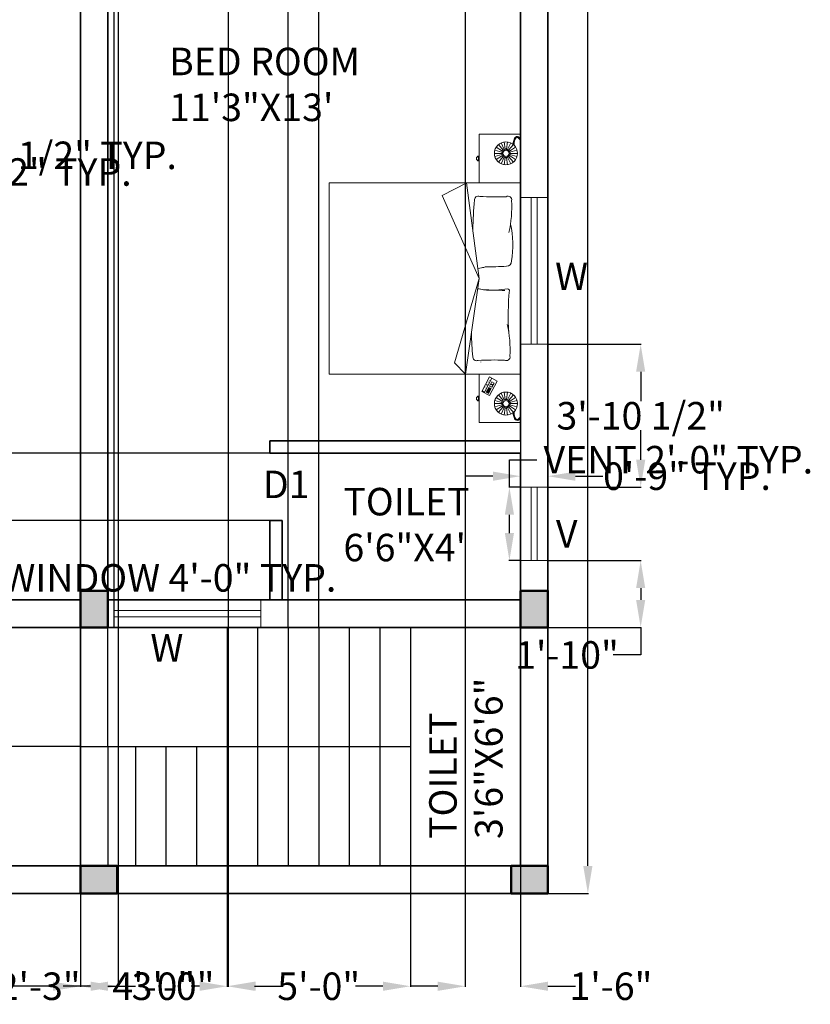
# Model space of a CAD drawing. Units: inches. Extents: x 113 to 575, y 111 to 799.
# Tile 2 of 4: x 317 to 575, y 119 to 441. Entities that reach past the tile are written whole.
import ezdxf

# ---------------------------------------------------------------- set-up
doc = ezdxf.new("R2010")
doc.units = ezdxf.units.IN
doc.header["$MEASUREMENT"] = 0
for name, color, linetype, lineweight in [('A-ANNO-DIMS', 2, 'Continuous', 18), ('A-ANNO-TEXT', 7, 'Continuous', 18), ('A-AREA-IDEN', 7, 'Continuous', 25), ('A-COLS', 7, 'Continuous', 50), ('A-COLS-PATT', 252, 'Continuous', 13), ('A-FLOR-STRS', 7, 'Continuous', 25), ('A-FURN', 8, 'Continuous', 18), ('A-GLAZ', 4, 'Continuous', 18), ('A-WALL', 7, 'Continuous', 35)]:
    doc.layers.add(name, color=color, linetype=linetype, lineweight=lineweight)
doc.styles.get("Standard").update_dxf_attribs({"font": 'arial.ttf'})
doc.dimstyles.get("Standard").update_dxf_attribs({"dimtxt": 9, "dimasz": 9, "dimexe": 0.18, "dimexo": 0.0625, "dimgap": 0.09, "dimtad": 0, "dimtih": 1, "dimtoh": 1, "dimdec": 0, "dimzin": 0, "dimdsep": 46, "dimlunit": 3, "dimtxsty": 'Standard', "dimcen": 0.09, "dimadec": 0, "dimazin": 0, "dimtfac": 1, "dimtdec": 0, "dimtofl": 0, "dimtmove": 0, "dimatfit": 3, "dimfxl": 1, "dimtolj": 1, "dimtzin": 0, "dimarcsym": 0})

# ---------------------------------------------------------------- blocks, each defined once
blk = doc.blocks.new('23')
for p, q in [((198.0513, 218.5507), (197.5897, 218.5507)), ((197.5897, 218.5507), (197.5897, 218.1608)), ((198.0513, 218.5507), (197.5897, 218.5507)), ((197.7114, 218.5049), (197.7492, 218.4461)), ((197.7398, 218.5179), (197.7595, 218.4508)), ((197.7707, 218.5223), (197.7707, 218.4524)), ((197.7707, 218.5223), (197.7707, 218.4524)), ((197.8016, 218.5179), (197.7819, 218.4508)), ((197.7922, 218.4461), (197.83, 218.5049)), ((198.0513, 216.7325), (198.0513, 218.5507)), ((198.0513, 218.5507), (198.9604, 218.5507)), ((198.0513, 218.5507), (199.8695, 218.5507)), ((198.0513, 218.5507), (198.0513, 218.1608)), ((199.8695, 218.5507), (200.3311, 218.5507)), ((199.8695, 218.5507), (200.3311, 218.5507)), ((199.8695, 218.5507), (199.8695, 216.7325)), ((200.1286, 218.4461), (200.0908, 218.5049)), ((200.1191, 218.5179), (200.1388, 218.4508)), ((200.15, 218.5223), (200.15, 218.4524)), ((200.15, 218.5223), (200.15, 218.4524)), ((200.1809, 218.5179), (200.1612, 218.4508)), ((200.2093, 218.5049), (200.1715, 218.4461)), ((200.3311, 218.5507), (200.3311, 218.1608)), ((197.6622, 218.4283), (197.7314, 218.4183)), ((197.6622, 218.3971), (197.7314, 218.407)), ((197.671, 218.4582), (197.7346, 218.4292)), ((197.671, 218.3671), (197.7346, 218.3962)), ((197.6878, 218.4845), (197.7407, 218.4387)), ((197.742, 218.419), (197.7324, 218.4232)), ((197.744, 218.425), (197.7336, 218.4267)), ((197.7863, 218.4377), (197.7953, 218.4438)), ((197.7934, 218.4314), (197.7991, 218.4404)), ((197.8007, 218.4387), (197.8536, 218.4845)), ((197.8068, 218.4292), (197.8704, 218.4582)), ((197.8068, 218.3962), (197.8704, 218.3671)), ((197.81, 218.4183), (197.8792, 218.4283)), ((197.81, 218.407), (197.8792, 218.3971)), ((200.1107, 218.4183), (200.0415, 218.4283)), ((200.1107, 218.407), (200.0415, 218.3971)), ((200.1139, 218.4292), (200.0503, 218.4582)), ((200.1139, 218.3962), (200.0503, 218.3671)), ((200.12, 218.4387), (200.0672, 218.4845)), ((200.1273, 218.4314), (200.1216, 218.4404)), ((200.1345, 218.4377), (200.1254, 218.4438)), ((200.1768, 218.425), (200.1872, 218.4267)), ((200.1788, 218.419), (200.1883, 218.4232)), ((200.2329, 218.4845), (200.18, 218.4387)), ((200.2498, 218.4582), (200.1862, 218.4292)), ((200.2498, 218.3671), (200.1862, 218.3962)), ((200.2586, 218.4283), (200.1893, 218.4183)), ((200.2586, 218.3971), (200.1893, 218.407)), ((197.6878, 218.3409), (197.7407, 218.3867)), ((197.7114, 218.3204), (197.7492, 218.3793)), ((197.7595, 218.3746), (197.7398, 218.3075)), ((197.7654, 218.3837), (197.7654, 218.3733)), ((197.7722, 218.3833), (197.7696, 218.373)), ((197.7707, 218.373), (197.7707, 218.303)), ((197.7707, 218.373), (197.7707, 218.303)), ((197.7819, 218.3746), (197.8016, 218.3075)), ((197.7922, 218.3793), (197.83, 218.3204)), ((197.8007, 218.3867), (197.8536, 218.3409)), ((199.897, 218.2553), (199.9365, 218.3298)), ((199.9365, 218.3298), (200.0738, 218.257)), ((200.12, 218.3867), (200.0672, 218.3409)), ((200.1286, 218.3793), (200.0908, 218.3204)), ((200.1388, 218.3746), (200.1191, 218.3075)), ((200.1486, 218.3833), (200.1512, 218.373)), ((200.15, 218.373), (200.15, 218.303)), ((200.15, 218.373), (200.15, 218.303)), ((200.1554, 218.3837), (200.1553, 218.3733)), ((200.1612, 218.3746), (200.1809, 218.3075)), ((200.2093, 218.3204), (200.1715, 218.3793)), ((200.2329, 218.3409), (200.18, 218.3867)), ((200.0344, 218.1825), (199.897, 218.2553)), ((199.9093, 218.2786), (200.0467, 218.2057)), ((199.9435, 218.2784), (199.9546, 218.2994)), ((199.9608, 218.2692), (199.9435, 218.2784)), ((199.9546, 218.2994), (199.972, 218.2902)), ((199.972, 218.2902), (199.9608, 218.2692)), ((199.9658, 218.2665), (199.977, 218.2875)), ((199.9832, 218.2573), (199.9658, 218.2665)), ((199.977, 218.2875), (199.9943, 218.2783)), ((199.9943, 218.2783), (199.9832, 218.2573)), ((199.9967, 218.2502), (200.0078, 218.2711)), ((200.0421, 218.2261), (199.9967, 218.2502)), ((200.044, 218.2298), (199.9986, 218.2538)), ((200.0458, 218.2332), (200.0004, 218.2572)), ((200.0469, 218.2353), (200.0016, 218.2594)), ((200.0482, 218.2378), (200.0029, 218.2618)), ((200.0498, 218.2406), (200.0044, 218.2647)), ((200.0519, 218.2446), (200.0065, 218.2687)), ((200.0532, 218.2471), (200.0078, 218.2711)), ((200.0738, 218.257), (200.0344, 218.1825)), ((200.0532, 218.2471), (200.0421, 218.2261)), ((197.5921, 218.1584), (198.0489, 218.1584)), ((197.7986, 218.1491), (197.7986, 218.1437)), ((197.84, 218.1515), (197.801, 218.1515)), ((197.801, 218.1413), (197.8052, 218.1413)), ((197.8076, 218.1389), (197.8076, 218.135)), ((197.81, 218.1326), (197.8309, 218.1326)), ((197.8286, 218.1584), (197.8124, 218.1584)), ((197.8124, 218.1584), (197.8124, 218.1515)), ((197.8286, 218.1515), (197.8286, 218.1584)), ((197.8333, 218.135), (197.8333, 218.1413)), ((197.8333, 218.1413), (197.84, 218.1413)), ((197.8424, 218.1437), (197.8424, 218.1491)), ((198.9604, 218.1582), (198.0513, 218.039)), ((198.171, 217.8058), (198.9604, 218.1582)), ((199.763, 217.9219), (198.9604, 218.1582)), ((198.9604, 218.1582), (199.8695, 218.0282)), ((200.3287, 218.1584), (199.8719, 218.1584)), ((200.0784, 218.1437), (200.0784, 218.1491)), ((200.0808, 218.1515), (200.1197, 218.1515)), ((200.0874, 218.1413), (200.0808, 218.1413)), ((200.0874, 218.135), (200.0874, 218.1413)), ((200.1107, 218.1326), (200.0898, 218.1326)), ((200.0922, 218.1515), (200.0922, 218.1584)), ((200.0922, 218.1584), (200.1084, 218.1584)), ((200.1084, 218.1584), (200.1084, 218.1515)), ((200.1131, 218.1389), (200.1131, 218.135)), ((200.1197, 218.1413), (200.1155, 218.1413)), ((200.1221, 218.1491), (200.1221, 218.1437)), ((198.0513, 218.042), (198.171, 217.8058)), ((199.8695, 218.0282), (199.763, 217.9219)), ((198.9604, 216.7325), (198.0513, 216.7325)), ((198.9604, 216.7325), (199.8695, 216.7325))]:
    blk.add_line(p, q)
for centre, radius in [((197.7707, 218.4127), 0.1096), ((200.15, 218.4127), 0.1096), ((197.7707, 218.4127), 0.0397), ((197.7707, 218.4127), 0.0294), ((200.15, 218.4127), 0.0397), ((200.15, 218.4127), 0.0294)]:
    blk.add_circle(centre, radius)
for centre, radius, start, end in [((198.2131, 218.4327), 0.035, 78.72779, 211.6095), ((198.2131, 218.4327), 0.035, 78.72779, 211.6095), ((194.5801, 218.3261), 3.6043, 357.43333, 1.40375), ((194.5801, 218.3261), 3.6043, 357.43333, 1.40375), ((198.2779, 217.3787), 1.0899, 77.05638, 93.04883), ((198.2779, 217.3787), 1.0899, 77.05638, 93.04883), ((198.6485, 217.4959), 0.982, 81.47023, 102.10326), ((198.6485, 217.4959), 0.982, 81.47023, 102.10326), ((198.7941, 218.4167), 0.0503, 0, 90), ((198.7941, 218.4167), 0.0503, 0, 90), ((192.8563, 218.1202), 5.9955, 0.91256, 2.83406), ((192.8563, 218.1202), 5.9955, 0.91256, 2.83406), ((199.1058, 218.4025), 0.0559, 128.22652, 148.49477), ((198.0818, 218.2709), 0.9895, 355.87807, 9.3556), ((205.0634, 218.1043), 5.9955, 177.16594, 179.08744), ((199.3105, 220.7603), 2.3262, 264.09622, 274.11018), ((199.1058, 218.4025), 0.0559, 41.3461, 41.8512), ((199.6418, 217.3627), 1.0899, 86.95117, 102.94362), ((199.6418, 217.3627), 1.0899, 86.95117, 102.94362), ((199.7066, 218.4167), 0.035, 328.3905, 101.27221), ((199.7066, 218.4167), 0.035, 328.3905, 101.27221), ((203.3397, 218.3101), 3.6043, 178.59625, 182.56667), ((203.3397, 218.3101), 3.6043, 178.59625, 182.56667), ((198.7853, 218.1859), 0.0722, 2.66977, 24.37437), ((198.5509, 218.1138), 0.3169, 5.86257, 18.75888), ((199.968, 218.2279), 0.00141, 90, 270), ((199.968, 218.2279), 0.00141, 270, 90), ((199.9724, 218.235), 0.00141, 90, 270), ((199.9724, 218.235), 0.00141, 270, 90), ((197.5921, 218.1608), 0.0024, 180, 270), ((197.801, 218.1491), 0.0024, 90, 180), ((197.801, 218.1437), 0.0024, 180, 270), ((197.8052, 218.1389), 0.0024, 0, 90), ((197.81, 218.135), 0.0024, 180, 270), ((197.8309, 218.135), 0.0024, 270, 0), ((197.84, 218.1491), 0.0024, 0, 90), ((197.84, 218.1437), 0.0024, 270, 0), ((198.2139, 218.15), 0.0362, 156.10841, 279.65758), ((198.2139, 218.15), 0.0362, 156.10841, 279.65758), ((198.5015, 220.904), 2.805, 264.11391, 269.91574), ((198.5015, 220.904), 2.805, 264.11391, 269.91574), ((199.1999, 218.1498), 0.1404, 159.16323, 182.37479), ((199.1345, 218.17), 0.0722, 155.62563, 177.33023), ((199.7059, 218.134), 0.0362, 260.34242, 23.89159), ((199.7059, 218.134), 0.0362, 260.34242, 23.89159), ((199.755, 218.1754), 0.00192, 180, 270), ((200.0315, 218.1913), 0.00141, 90, 270), ((200.0315, 218.1913), 0.00141, 270, 90), ((200.0366, 218.2002), 0.00141, 90, 270), ((200.0366, 218.2002), 0.00141, 270, 90), ((200.0808, 218.1491), 0.0024, 90, 180), ((200.0808, 218.1437), 0.0024, 180, 270), ((200.0898, 218.135), 0.0024, 180, 270), ((200.1107, 218.135), 0.0024, 270, 0), ((200.1155, 218.1389), 0.0024, 90, 180), ((200.1197, 218.1491), 0.0024, 0, 90), ((200.1197, 218.1437), 0.0024, 270, 0), ((200.3287, 218.1608), 0.0024, 270, 0), ((199.4182, 220.888), 2.805, 271.28421, 275.88609), ((199.4182, 220.888), 2.805, 271.28421, 275.88609)]:
    blk.add_arc(centre, radius, start, end)
for points, knots in [([(197.6859, 218.4822), (197.6739, 218.4821), (197.6612, 218.4826), (197.6341, 218.4911), (197.617, 218.4975), (197.6078, 218.5268), (197.618, 218.5375), (197.6293, 218.5478), (197.6309, 218.5493), (197.6326, 218.5507)], [0.0077183, 0.0077183, 0.0077183, 0.0077183, 0.0428867, 0.0428867, 0.0785443, 0.0785443, 0.1084778, 0.1084778, 0.1132873, 0.1132873, 0.1132873, 0.1132873]), ([(197.6936, 218.4906), (197.6769, 218.4903), (197.6508, 218.4898), (197.6068, 218.5187), (197.631, 218.5387), (197.6455, 218.5507)], [0, 0, 0, 0, 0.0514038, 0.0806942, 0.123773, 0.123773, 0.123773, 0.123773]), ([(200.2272, 218.4906), (200.2438, 218.4903), (200.2699, 218.4898), (200.3139, 218.5187), (200.2897, 218.5387), (200.2753, 218.5507)], [0, 0, 0, 0, 0.0514038, 0.0806942, 0.123773, 0.123773, 0.123773, 0.123773]), ([(200.2348, 218.4822), (200.2468, 218.4821), (200.2595, 218.4826), (200.2866, 218.4911), (200.3037, 218.4975), (200.3129, 218.5268), (200.3027, 218.5375), (200.2914, 218.5478), (200.2898, 218.5493), (200.2882, 218.5507)], [0.0077183, 0.0077183, 0.0077183, 0.0077183, 0.0428867, 0.0428867, 0.0785443, 0.0785443, 0.1084778, 0.1084778, 0.1132873, 0.1132873, 0.1132873, 0.1132873])]:
    blk.add_open_spline(points, degree=3, knots=knots)
at = {"width": 3}
blk.add_text('12 00', height=0.01005, rotation=330.64352, dxfattribs=at).set_placement((199.9154, 218.2567))
blk = doc.blocks.new('*D7')
at = {"layer": 'A-ANNO-DIMS', "color": 0, "lineweight": -2, "transparency": 16777216}
for p, q in [((489.56, 754.81), (502.74, 754.81)), ((502.56, 745.81), (502.56, 459.5)), ((502.56, 163.81), (502.56, 450.13)), ((489.56, 154.81), (502.74, 154.81))]:
    blk.add_line(p, q, dxfattribs=at)
at = {"layer": 'A-ANNO-DIMS', "color": 0, "transparency": 16777216}
for points in [[(501.06, 745.81), (504.06, 745.81), (502.56, 754.81)], [(501.06, 163.81), (504.06, 163.81), (502.56, 154.81)]]:
    blk.add_solid(points, dxfattribs=at)
at = {"layer": 'Defpoints', "color": 0, "transparency": 16777216}
for p in [(489.49, 754.81), (489.49, 154.81), (502.56, 154.81)]:
    blk.add_point(p, dxfattribs=at)
at = {"layer": 'A-ANNO-DIMS', "color": 0, "transparency": 16777216, "insert": (502.56, 454.81), "char_height": 9, "attachment_point": 5}
blk.add_mtext("\\A1;50'", dxfattribs=at)
blk = doc.blocks.new('WIN-48IN')
for p, q in [((0, 9), (0, 0)), ((48, 9), (48, 0)), ((0, 5.5), (48, 5.5)), ((0, 3.5), (48, 3.5))]:
    blk.add_line(p, q)
blk = doc.blocks.new('VENT-24IN')
for p, q in [((0, 24), (9, 24)), ((3.5, 0), (3.5, 24)), ((5.5, 0), (5.5, 24)), ((0, 0), (9, 0))]:
    blk.add_line(p, q)
blk = doc.blocks.new('*D10')
at = {"layer": 'A-ANNO-DIMS', "color": 0, "lineweight": -2, "transparency": 16777216}
for p, q in [((251.58, 250.88), (251.58, 258.19)), ((260.58, 258.01), (290.58, 258.01)), ((299.58, 250.88), (299.58, 258.19)), ((299.58, 258.01), (308.58, 258.01))]:
    blk.add_line(p, q, dxfattribs=at)
at = {"layer": 'A-ANNO-DIMS', "color": 0, "transparency": 16777216}
for points in [[(260.58, 259.51), (260.58, 256.51), (251.58, 258.01)], [(290.58, 259.51), (290.58, 256.51), (299.58, 258.01)]]:
    blk.add_solid(points, dxfattribs=at)
at = {"layer": 'Defpoints', "color": 0, "transparency": 16777216}
for p in [(299.58, 258.01), (251.58, 250.81), (299.58, 250.81)]:
    blk.add_point(p, dxfattribs=at)
at = {"layer": 'A-ANNO-DIMS', "color": 0, "transparency": 16777216, "insert": (365.61, 258.01), "char_height": 9, "attachment_point": 5}
blk.add_mtext('\\A1;WINDOW 4\'-0" TYP.', dxfattribs=at)
blk = doc.blocks.new('*D12')
at = {"layer": 'A-ANNO-DIMS', "color": 0, "lineweight": -2, "transparency": 16777216}
for p, q in [((476.89, 287.66), (476.89, 296.66)), ((476.89, 296.66), (485.89, 296.66)), ((480.43, 287.66), (476.71, 287.66)), ((476.89, 272.66), (476.89, 278.66)), ((480.43, 263.66), (476.71, 263.66))]:
    blk.add_line(p, q, dxfattribs=at)
at = {"layer": 'A-ANNO-DIMS', "color": 0, "transparency": 16777216}
for points in [[(475.39, 278.66), (478.39, 278.66), (476.89, 287.66)], [(475.39, 272.66), (478.39, 272.66), (476.89, 263.66)]]:
    blk.add_solid(points, dxfattribs=at)
at = {"layer": 'Defpoints', "color": 0, "transparency": 16777216}
for p in [(476.89, 287.66), (480.49, 287.66), (480.49, 263.66)]:
    blk.add_point(p, dxfattribs=at)
at = {"layer": 'A-ANNO-DIMS', "color": 0, "transparency": 16777216, "insert": (532.16, 296.66), "char_height": 9, "attachment_point": 5}
blk.add_mtext('\\A1;VENT 2\'-0" TYP.', dxfattribs=at)
blk = doc.blocks.new('*D13')
at = {"layer": 'A-ANNO-DIMS', "color": 0, "lineweight": -2, "transparency": 16777216}
for p, q in [((471.49, 291.26), (462.49, 291.26)), ((480.49, 287.72), (480.49, 291.44)), ((489.49, 287.72), (489.49, 291.44)), ((498.49, 291.26), (507.49, 291.26))]:
    blk.add_line(p, q, dxfattribs=at)
at = {"layer": 'A-ANNO-DIMS', "color": 0, "transparency": 16777216}
for points in [[(471.49, 292.76), (471.49, 289.76), (480.49, 291.26)], [(498.49, 292.76), (498.49, 289.76), (489.49, 291.26)]]:
    blk.add_solid(points, dxfattribs=at)
at = {"layer": 'Defpoints', "color": 0, "transparency": 16777216}
for p in [(489.49, 291.26), (480.49, 287.66), (489.49, 287.66)]:
    blk.add_point(p, dxfattribs=at)
at = {"layer": 'A-ANNO-DIMS', "color": 0, "transparency": 16777216, "insert": (535.01, 291.26), "char_height": 9, "attachment_point": 5}
blk.add_mtext('\\A1;0\'-9" TYP.', dxfattribs=at)
blk = doc.blocks.new('*D16')
at = {"layer": 'A-ANNO-DIMS', "color": 0, "lineweight": -2, "transparency": 16777216}
for p, q in [((234.56, 387.2), (234.56, 396.2)), ((234.56, 396.2), (243.56, 396.2)), ((238.04, 387.2), (234.38, 387.2)), ((234.56, 372.58), (234.56, 378.2)), ((238.04, 363.58), (234.38, 363.58))]:
    blk.add_line(p, q, dxfattribs=at)
at = {"layer": 'A-ANNO-DIMS', "color": 0, "transparency": 16777216}
for points in [[(233.06, 378.2), (236.06, 378.2), (234.56, 387.2)], [(233.06, 372.58), (236.06, 372.58), (234.56, 363.58)]]:
    blk.add_solid(points, dxfattribs=at)
at = {"layer": 'Defpoints', "color": 0, "transparency": 16777216}
for p in [(234.56, 387.2), (238.1, 387.2), (238.1, 363.58)]:
    blk.add_point(p, dxfattribs=at)
at = {"layer": 'A-ANNO-DIMS', "color": 0, "transparency": 16777216, "insert": (306.83, 396.2), "char_height": 9, "attachment_point": 5}
blk.add_mtext('\\A1;TABLE 1\'-11 1/2" TYP.', dxfattribs=at)
blk = doc.blocks.new('*D17')
at = {"layer": 'A-ANNO-DIMS', "color": 0, "lineweight": -2, "transparency": 16777216}
for p, q in [((238.1, 387.26), (238.1, 390.92)), ((247.1, 390.74), (252.72, 390.74)), ((261.72, 387.26), (261.72, 390.92)), ((261.72, 390.74), (270.72, 390.74))]:
    blk.add_line(p, q, dxfattribs=at)
at = {"layer": 'A-ANNO-DIMS', "color": 0, "transparency": 16777216}
for points in [[(247.1, 392.24), (247.1, 389.24), (238.1, 390.74)], [(252.72, 392.24), (252.72, 389.24), (261.72, 390.74)]]:
    blk.add_solid(points, dxfattribs=at)
at = {"layer": 'Defpoints', "color": 0, "transparency": 16777216}
for p in [(261.72, 390.74), (238.1, 387.2), (261.72, 387.2)]:
    blk.add_point(p, dxfattribs=at)
at = {"layer": 'A-ANNO-DIMS', "color": 0, "transparency": 16777216, "insert": (311.8, 390.74), "char_height": 9, "attachment_point": 5}
blk.add_mtext('\\A1;1\'-11 1/2" TYP.', dxfattribs=at)
blk = doc.blocks.new('*D22')
at = {"layer": 'A-ANNO-DIMS', "color": 0, "lineweight": -2, "transparency": 16777216}
for p, q in [((177.49, 154.75), (177.49, 124.27)), ((336.49, 154.75), (336.49, 124.27)), ((186.49, 124.45), (241.87, 124.45)), ((327.49, 124.45), (272.12, 124.45))]:
    blk.add_line(p, q, dxfattribs=at)
at = {"layer": 'A-ANNO-DIMS', "color": 0, "transparency": 16777216}
for points in [[(186.49, 125.95), (186.49, 122.95), (177.49, 124.45)], [(327.49, 125.95), (327.49, 122.95), (336.49, 124.45)]]:
    blk.add_solid(points, dxfattribs=at)
at = {"layer": 'Defpoints', "color": 0, "transparency": 16777216}
for p in [(177.49, 154.81), (336.49, 154.81), (336.49, 124.45)]:
    blk.add_point(p, dxfattribs=at)
at = {"layer": 'A-ANNO-DIMS', "color": 0, "transparency": 16777216, "insert": (256.99, 124.45), "char_height": 9, "attachment_point": 5}
blk.add_mtext('\\A1;13\'-3"', dxfattribs=at)
blk = doc.blocks.new('*D23')
at = {"layer": 'A-ANNO-DIMS', "color": 0, "lineweight": -2, "transparency": 16777216}
for p, q in [((336.49, 163.75), (336.49, 124.27)), ((384.49, 163.75), (384.49, 124.27)), ((345.49, 124.45), (348.26, 124.45)), ((375.49, 124.45), (372.73, 124.45))]:
    blk.add_line(p, q, dxfattribs=at)
at = {"layer": 'A-ANNO-DIMS', "color": 0, "transparency": 16777216}
for points in [[(345.49, 125.95), (345.49, 122.95), (336.49, 124.45)], [(375.49, 125.95), (375.49, 122.95), (384.49, 124.45)]]:
    blk.add_solid(points, dxfattribs=at)
at = {"layer": 'Defpoints', "color": 0, "transparency": 16777216}
for p in [(336.49, 163.81), (384.49, 163.81), (384.49, 124.45)]:
    blk.add_point(p, dxfattribs=at)
at = {"layer": 'A-ANNO-DIMS', "color": 0, "transparency": 16777216, "insert": (360.49, 124.45), "char_height": 9, "attachment_point": 5}
blk.add_mtext('\\A1;4\'-0"', dxfattribs=at)
blk = doc.blocks.new('*D24')
at = {"layer": 'A-ANNO-DIMS', "color": 0, "lineweight": -2, "transparency": 16777216}
for p, q in [((384.49, 163.75), (384.49, 124.27)), ((444.49, 163.75), (444.49, 124.27)), ((393.49, 124.45), (402.44, 124.45)), ((435.49, 124.45), (426.55, 124.45))]:
    blk.add_line(p, q, dxfattribs=at)
at = {"layer": 'A-ANNO-DIMS', "color": 0, "transparency": 16777216}
for points in [[(393.49, 125.95), (393.49, 122.95), (384.49, 124.45)], [(435.49, 125.95), (435.49, 122.95), (444.49, 124.45)]]:
    blk.add_solid(points, dxfattribs=at)
at = {"layer": 'Defpoints', "color": 0, "transparency": 16777216}
for p in [(384.49, 163.81), (444.49, 163.81), (444.49, 124.45)]:
    blk.add_point(p, dxfattribs=at)
at = {"layer": 'A-ANNO-DIMS', "color": 0, "transparency": 16777216, "insert": (414.49, 124.45), "char_height": 9, "attachment_point": 5}
blk.add_mtext('\\A1;5\'-0"', dxfattribs=at)
blk = doc.blocks.new('*D25')
at = {"layer": 'A-ANNO-DIMS', "color": 0, "lineweight": -2, "transparency": 16777216}
for p, q in [((336.43, 202.81), (146.96, 202.81)), ((147.14, 193.81), (147.14, 188)), ((147.14, 172.81), (147.14, 178.62)), ((336.43, 163.81), (146.96, 163.81))]:
    blk.add_line(p, q, dxfattribs=at)
at = {"layer": 'A-ANNO-DIMS', "color": 0, "transparency": 16777216}
for points in [[(145.64, 193.81), (148.64, 193.81), (147.14, 202.81)], [(145.64, 172.81), (148.64, 172.81), (147.14, 163.81)]]:
    blk.add_solid(points, dxfattribs=at)
at = {"layer": 'Defpoints', "color": 0, "transparency": 16777216}
for p in [(147.14, 202.81), (336.49, 202.81), (336.49, 163.81)]:
    blk.add_point(p, dxfattribs=at)
at = {"layer": 'A-ANNO-DIMS', "color": 0, "transparency": 16777216, "insert": (147.14, 183.31), "char_height": 9, "attachment_point": 5}
blk.add_mtext('\\A1;3\'-3"', dxfattribs=at)
blk = doc.blocks.new('*D26')
at = {"layer": 'A-ANNO-DIMS', "color": 0, "lineweight": -2, "transparency": 16777216}
for p, q in [((395.49, 785.17), (386.49, 785.17)), ((404.49, 241.88), (404.49, 785.35)), ((414.49, 241.88), (414.49, 785.35)), ((423.49, 785.17), (432.49, 785.17))]:
    blk.add_line(p, q, dxfattribs=at)
at = {"layer": 'A-ANNO-DIMS', "color": 0, "transparency": 16777216}
for points in [[(395.49, 786.67), (395.49, 783.67), (404.49, 785.17)], [(423.49, 786.67), (423.49, 783.67), (414.49, 785.17)]]:
    blk.add_solid(points, dxfattribs=at)
at = {"layer": 'Defpoints', "color": 0, "transparency": 16777216}
for p in [(414.49, 785.17), (404.49, 241.81), (414.49, 241.81)]:
    blk.add_point(p, dxfattribs=at)
at = {"layer": 'A-ANNO-DIMS', "color": 0, "transparency": 16777216, "insert": (448.04, 785.17), "char_height": 9, "attachment_point": 5}
blk.add_mtext('\\A1;0\'-10"', dxfattribs=at)
blk = doc.blocks.new('*D27')
at = {"layer": 'A-ANNO-DIMS', "color": 0, "lineweight": -2, "transparency": 16777216}
for p, q in [((327.49, 785.17), (318.49, 785.17)), ((336.49, 202.88), (336.49, 785.35)), ((345.49, 202.88), (345.49, 785.35)), ((354.49, 785.17), (363.49, 785.17))]:
    blk.add_line(p, q, dxfattribs=at)
at = {"layer": 'A-ANNO-DIMS', "color": 0, "transparency": 16777216}
for points in [[(327.49, 786.67), (327.49, 783.67), (336.49, 785.17)], [(354.49, 786.67), (354.49, 783.67), (345.49, 785.17)]]:
    blk.add_solid(points, dxfattribs=at)
at = {"layer": 'Defpoints', "color": 0, "transparency": 16777216}
for p in [(345.49, 785.17), (336.49, 202.81), (345.49, 202.81)]:
    blk.add_point(p, dxfattribs=at)
at = {"layer": 'A-ANNO-DIMS', "color": 0, "transparency": 16777216, "insert": (375.55, 785.17), "char_height": 9, "attachment_point": 5}
blk.add_mtext('\\A1;0\'-9"', dxfattribs=at)
blk = doc.blocks.new('*D32')
at = {"layer": 'A-ANNO-DIMS', "color": 0, "lineweight": -2, "transparency": 16777216}
for p, q in [((480.49, 601.75), (480.49, 124.27)), ((462.45, 597.75), (462.45, 124.27)), ((453.45, 124.45), (444.45, 124.45)), ((489.49, 124.45), (498.49, 124.45))]:
    blk.add_line(p, q, dxfattribs=at)
at = {"layer": 'A-ANNO-DIMS', "color": 0, "transparency": 16777216}
for points in [[(453.45, 125.95), (453.45, 122.95), (462.45, 124.45)], [(489.49, 125.95), (489.49, 122.95), (480.49, 124.45)]]:
    blk.add_solid(points, dxfattribs=at)
at = {"layer": 'Defpoints', "color": 0, "transparency": 16777216}
for p in [(480.49, 601.81), (462.45, 597.81), (480.49, 124.45)]:
    blk.add_point(p, dxfattribs=at)
at = {"layer": 'A-ANNO-DIMS', "color": 0, "transparency": 16777216, "insert": (510.12, 124.45), "char_height": 9, "attachment_point": 5}
blk.add_mtext('\\A1;1\'-6"', dxfattribs=at)
blk = doc.blocks.new('*D33')
at = {"layer": 'A-ANNO-DIMS', "color": 0, "lineweight": -2, "transparency": 16777216}
for p, q in [((147.14, 298.81), (147.14, 307.81)), ((147.14, 307.81), (156.14, 307.81)), ((398.43, 298.81), (146.96, 298.81)), ((147.14, 285.81), (147.14, 289.81)), ((398.43, 276.81), (146.96, 276.81))]:
    blk.add_line(p, q, dxfattribs=at)
at = {"layer": 'A-ANNO-DIMS', "color": 0, "transparency": 16777216}
for points in [[(145.64, 289.81), (148.64, 289.81), (147.14, 298.81)], [(145.64, 285.81), (148.64, 285.81), (147.14, 276.81)]]:
    blk.add_solid(points, dxfattribs=at)
at = {"layer": 'Defpoints', "color": 0, "transparency": 16777216}
for p in [(147.14, 298.81), (398.49, 298.81), (398.49, 276.81)]:
    blk.add_point(p, dxfattribs=at)
at = {"layer": 'A-ANNO-DIMS', "color": 0, "transparency": 16777216, "insert": (171.26, 307.81), "char_height": 9, "attachment_point": 5}
blk.add_mtext('\\A1;1\'-10"', dxfattribs=at)
blk = doc.blocks.new('*D38')
at = {"layer": 'A-ANNO-DIMS', "color": 0, "lineweight": -2, "transparency": 16777216}
for p, q in [((489.56, 263.66), (520.03, 263.66)), ((519.85, 254.66), (519.85, 250.81)), ((489.56, 241.81), (520.03, 241.81)), ((519.85, 241.81), (519.85, 232.81)), ((519.85, 232.81), (510.85, 232.81))]:
    blk.add_line(p, q, dxfattribs=at)
at = {"layer": 'A-ANNO-DIMS', "color": 0, "transparency": 16777216}
for points in [[(518.35, 254.66), (521.35, 254.66), (519.85, 263.66)], [(518.35, 250.81), (521.35, 250.81), (519.85, 241.81)]]:
    blk.add_solid(points, dxfattribs=at)
at = {"layer": 'Defpoints', "color": 0, "transparency": 16777216}
for p in [(489.49, 263.66), (489.49, 241.81), (519.85, 241.81)]:
    blk.add_point(p, dxfattribs=at)
at = {"layer": 'A-ANNO-DIMS', "color": 0, "transparency": 16777216, "insert": (495.73, 232.81), "char_height": 9, "attachment_point": 5}
blk.add_mtext('\\A1;1\'-10"', dxfattribs=at)
blk = doc.blocks.new('*D39')
at = {"layer": 'A-ANNO-DIMS', "color": 0, "lineweight": -2, "transparency": 16777216}
for p, q in [((489.56, 334.4), (520.03, 334.4)), ((519.85, 325.4), (519.85, 315.78)), ((519.85, 296.66), (519.85, 306.28)), ((489.56, 287.66), (520.03, 287.66))]:
    blk.add_line(p, q, dxfattribs=at)
at = {"layer": 'A-ANNO-DIMS', "color": 0, "transparency": 16777216}
for points in [[(518.35, 325.4), (521.35, 325.4), (519.85, 334.4)], [(518.35, 296.66), (521.35, 296.66), (519.85, 287.66)]]:
    blk.add_solid(points, dxfattribs=at)
at = {"layer": 'Defpoints', "color": 0, "transparency": 16777216}
for p in [(489.49, 334.4), (519.85, 334.4), (489.49, 287.66)]:
    blk.add_point(p, dxfattribs=at)
at = {"layer": 'A-ANNO-DIMS', "color": 0, "transparency": 16777216, "insert": (519.85, 311.03), "char_height": 9, "attachment_point": 5}
blk.add_mtext('\\A1;3\'-10 1/2"', dxfattribs=at)
blk = doc.blocks.new('*D43')
at = {"layer": 'A-ANNO-DIMS', "color": 0, "lineweight": -2, "transparency": 16777216}
for p, q in [((336.49, 785.17), (327.49, 785.17)), ((345.49, 241.88), (345.49, 785.35)), ((347.52, 241.88), (347.52, 785.35)), ((356.52, 785.17), (365.52, 785.17))]:
    blk.add_line(p, q, dxfattribs=at)
at = {"layer": 'A-ANNO-DIMS', "color": 0, "transparency": 16777216}
for points in [[(336.49, 786.67), (336.49, 783.67), (345.49, 785.17)], [(356.52, 786.67), (356.52, 783.67), (347.52, 785.17)]]:
    blk.add_solid(points, dxfattribs=at)
at = {"layer": 'Defpoints', "color": 0, "transparency": 16777216}
for p in [(347.52, 785.17), (345.49, 241.81), (347.52, 241.81)]:
    blk.add_point(p, dxfattribs=at)
at = {"layer": 'A-ANNO-DIMS', "color": 0, "transparency": 16777216, "insert": (377.57, 785.17), "char_height": 9, "attachment_point": 5}
blk.add_mtext('\\A1;0\'-2"', dxfattribs=at)
blk = doc.blocks.new('*D47')
at = {"layer": 'A-ANNO-DIMS', "color": 0, "lineweight": -2, "transparency": 16777216}
for p, q in [((348.815003, 460.750317), (348.815003, 124.273067)), ((384.815003, 460.750317), (384.815003, 124.273067)), ((339.815003, 124.453067), (330.815003, 124.453067)), ((393.815003, 124.453067), (402.815003, 124.453067))]:
    blk.add_line(p, q, dxfattribs=at)
at = {"layer": 'A-ANNO-DIMS', "color": 0, "transparency": 16777216}
for points in [[(339.815003, 125.953067), (339.815003, 122.953067), (348.815003, 124.453067)], [(393.815003, 125.953067), (393.815003, 122.953067), (384.815003, 124.453067)]]:
    blk.add_solid(points, dxfattribs=at)
at = {"layer": 'Defpoints', "color": 0, "transparency": 16777216}
for p in [(348.815003, 460.812817), (384.815003, 460.812817), (384.815003, 124.453067)]:
    blk.add_point(p, dxfattribs=at)
at = {"layer": 'A-ANNO-DIMS', "color": 0, "transparency": 16777216, "insert": (366.815003, 124.453067), "char_height": 9, "attachment_point": 5}
blk.add_mtext('\\A1;3\'-0"', dxfattribs=at)
blk = doc.blocks.new('*D49')
at = {"layer": 'A-ANNO-DIMS', "color": 0, "lineweight": -2, "transparency": 16777216}
for p, q in [((309.494828, 592.750317), (309.494828, 124.273067)), ((336.494828, 592.750317), (336.494828, 124.273067)), ((300.494828, 124.453067), (291.494828, 124.453067)), ((345.494828, 124.453067), (354.494828, 124.453067))]:
    blk.add_line(p, q, dxfattribs=at)
at = {"layer": 'A-ANNO-DIMS', "color": 0, "transparency": 16777216}
for points in [[(300.494828, 125.953067), (300.494828, 122.953067), (309.494828, 124.453067)], [(345.494828, 125.953067), (345.494828, 122.953067), (336.494828, 124.453067)]]:
    blk.add_solid(points, dxfattribs=at)
at = {"layer": 'Defpoints', "color": 0, "transparency": 16777216}
for p in [(309.494828, 592.812817), (336.494828, 592.812817), (336.494828, 124.453067)]:
    blk.add_point(p, dxfattribs=at)
at = {"layer": 'A-ANNO-DIMS', "color": 0, "transparency": 16777216, "insert": (322.994828, 124.453067), "char_height": 9, "attachment_point": 5}
blk.add_mtext('\\A1;2\'-3"', dxfattribs=at)

msp = doc.modelspace()

# ---------------------------------------------------------------- hatches: boundary and pattern name
at = {"layer": 'A-COLS-PATT'}
h = msp.add_hatch(color=256, dxfattribs=at)
h.dxf.hatch_style = 1
h.paths.add_polyline_path([(186.49, 754.81), (177.49, 754.81), (177.49, 742.81), (186.49, 742.81)])
h.paths.add_polyline_path([(345.49, 754.81), (336.49, 754.81), (336.49, 742.81), (345.49, 742.81)])
h.paths.add_polyline_path([(489.49, 754.81), (480.49, 754.81), (480.49, 742.81), (489.49, 742.81)])
h.paths.add_polyline_path([(489.49, 601.81), (480.49, 601.81), (480.49, 589.81), (489.49, 589.81)])
h.paths.add_polyline_path([(345.49, 604.81), (336.49, 604.81), (336.49, 592.81), (345.49, 592.81)])
h.paths.add_polyline_path([(186.49, 604.81), (177.49, 604.81), (177.49, 592.81), (186.49, 592.81)])
h.paths.add_polyline_path([(186.49, 472.81), (177.49, 472.81), (177.49, 460.81), (186.49, 460.81)])
h.paths.add_polyline_path([(345.49, 469.81), (336.49, 469.81), (336.49, 457.81), (345.49, 457.81)])
h.paths.add_polyline_path([(489.49, 469.81), (480.49, 469.81), (480.49, 457.81), (489.49, 457.81)])
h.paths.add_polyline_path([(186.49, 253.81), (177.49, 253.81), (177.49, 241.81), (186.49, 241.81)])
h.paths.add_polyline_path([(345.49, 253.81), (336.49, 253.81), (336.49, 241.81), (345.49, 241.81)])
h.paths.add_polyline_path([(489.49, 253.81), (480.49, 253.81), (480.49, 241.81), (489.49, 241.81)])
h.paths.add_polyline_path([(489.49, 163.81), (477.49, 163.81), (477.49, 154.81), (489.49, 154.81)])
h.paths.add_polyline_path([(348.49, 163.81), (336.49, 163.81), (336.49, 154.81), (348.49, 154.81)])
h.paths.add_polyline_path([(189.49, 163.81), (177.49, 163.81), (177.49, 154.81), (189.49, 154.81)])

# ---------------------------------------------------------------- linework, layer by layer
at = {"layer": 'A-COLS'}
for points in [[(336.49, 253.81), (345.49, 253.81), (345.49, 241.81), (336.49, 241.81)], [(480.49, 253.81), (489.49, 253.81), (489.49, 241.81), (480.49, 241.81)], [(336.49, 154.81), (336.49, 163.81), (348.49, 163.81), (348.49, 154.81)], [(477.49, 154.81), (477.49, 163.81), (489.49, 163.81), (489.49, 154.81)]]:
    msp.add_lwpolyline(points, close=True, dxfattribs=at)
at = {"layer": 'A-FLOR-STRS'}
for p, q in [((384.49, 241.81), (384.49, 163.81)), ((394.49, 241.81), (394.49, 163.81)), ((404.49, 241.81), (404.49, 163.81)), ((414.49, 241.81), (414.49, 163.81)), ((424.49, 241.81), (424.49, 163.81)), ((434.49, 241.81), (434.49, 163.81)), ((444.49, 241.81), (444.49, 163.81)), ((336.49, 163.81), (336.49, 202.81)), ((336.49, 202.81), (444.49, 202.81)), ((345.49, 202.81), (345.49, 163.81)), ((354.49, 202.81), (354.49, 163.81)), ((364.49, 202.81), (364.49, 163.81)), ((374.49, 202.81), (374.49, 163.81))]:
    msp.add_line(p, q, dxfattribs=at)
at = {"layer": 'A-WALL'}
for p, q in [((489.49, 754.81), (489.49, 154.81)), ((480.49, 544.81), (480.49, 302.81)), ((336.49, 241.81), (336.49, 475.62)), ((345.49, 475.62), (345.49, 241.81)), ((398.49, 302.81), (480.49, 302.81)), ((398.49, 302.81), (398.49, 298.81)), ((398.49, 298.81), (480.49, 298.81)), ((480.49, 298.81), (480.49, 163.81)), ((398.49, 276.81), (402.49, 276.81)), ((398.49, 276.81), (398.49, 250.81)), ((402.49, 276.81), (402.49, 250.81)), ((238.28, 250.81), (336.49, 250.81)), ((345.49, 250.81), (480.49, 250.81)), ((238.28, 241.81), (480.49, 241.81)), ((480.49, 163.81), (186.49, 163.81)), ((489.49, 154.81), (177.49, 154.81))]:
    msp.add_line(p, q, dxfattribs=at)

# ---------------------------------------------------------------- block references
at = {"layer": 'A-FURN', "xscale": 34.39932596969199, "yscale": 34.39932596969199, "zscale": 34.39932596969199, "rotation": 270}
msp.add_blockref('23', (-7037.5, 7200.03), dxfattribs=at)
at = {"layer": 'A-GLAZ', "rotation": 90.00000000000011}
msp.add_blockref('WIN-48IN', (489.49, 334.4), dxfattribs=at)
at = {"layer": 'A-GLAZ'}
for name, p in [('VENT-24IN', (480.49, 263.66)), ('WIN-48IN', (347.52, 241.81))]:
    msp.add_blockref(name, p, dxfattribs=at)

# ---------------------------------------------------------------- texts
at = {"layer": 'A-ANNO-TEXT', "char_height": 9, "attachment_point": 1}
for s, insert in [('W', (491.84, 361.13)), ('D1', (396.22, 293.08)), ('V', (492.11, 276.93)), ('W', (359.4, 239.61))]:
    msp.add_mtext_dynamic_manual_height_columns(s, width=17.4228, gutter_width=1, heights=[0], dxfattribs=dict(at, insert=insert))
at = {"layer": 'A-AREA-IDEN', "char_height": 9, "attachment_point": 1}
for s, insert in [('BED ROOM\\P11\'3"X13\'', (365.52, 431.4)), ('TOILET\\P6\'6"X4\'', (422.56, 287.44))]:
    msp.add_mtext_dynamic_manual_height_columns(s, width=130.397, gutter_width=1, heights=[0], dxfattribs=dict(at, insert=insert))
at = {"layer": 'A-AREA-IDEN', "insert": (450.64, 172.62), "char_height": 9, "attachment_point": 1, "rotation": 90}
msp.add_mtext_dynamic_manual_height_columns('TOILET\\P3\'6"X6\'6"', width=130.397, gutter_width=1, heights=[0], dxfattribs=at)

# ---------------------------------------------------------------- dimensions: what is measured, and where the dimension line sits
at = {"layer": 'A-ANNO-DIMS'}
for base, p1, p2, picture, middle in [((345.49, 785.17), (336.49, 202.81), (345.49, 202.81), '*D27', (375.55, 785.17)), ((347.52, 785.17), (345.49, 241.81), (347.52, 241.81), '*D43', (377.57, 785.17)), ((414.49, 785.17), (404.49, 241.81), (414.49, 241.81), '*D26', (448.04, 785.17)), ((480.49, 124.45), (462.45, 597.81), (480.49, 601.81), '*D32', (510.12, 124.45)), ((336.49, 124.45), (309.49, 592.81), (336.49, 592.81), '*D49', (322.99, 124.45)), ((384.82, 124.45), (348.82, 460.81), (384.82, 460.81), '*D47', (366.82, 124.45)), ((384.49, 124.45), (336.49, 163.81), (384.49, 163.81), '*D23', (360.49, 124.45)), ((444.49, 124.45), (384.49, 163.81), (444.49, 163.81), '*D24', (414.49, 124.45)), ((336.49, 124.45), (177.49, 154.81), (336.49, 154.81), '*D22', (256.99, 124.45))]:
    dim = msp.add_linear_dim(base=base, p1=p1, p2=p2, dimstyle='Standard', override={"dimdec": 1, "dimlfac": 1, "dimrnd": 0, "dimzin": 1, "dimdsep": 46, "dimlunit": 4, "dimfrac": 2}, dxfattribs=at)
    dim.commit()
    dim.dimension.update_dxf_attribs({"geometry": picture, "text_midpoint": middle})
for base, p1, p2, override, picture, middle in [((502.56, 154.81), (489.49, 754.81), (489.49, 154.81), {"dimclrd": 0, "dimclre": 0, "dimclrt": 0}, '*D7', (502.56, 454.81)), ((519.85, 334.4), (489.49, 287.66), (489.49, 334.4), {"dimdec": 1, "dimlfac": 1, "dimrnd": 0, "dimzin": 1, "dimdsep": 46, "dimlunit": 4, "dimfrac": 2}, '*D39', (519.85, 311.03)), ((147.14, 298.81), (398.49, 276.81), (398.49, 298.81), {"dimdec": 1, "dimlfac": 1, "dimrnd": 0, "dimzin": 1, "dimdsep": 46, "dimlunit": 4, "dimfrac": 2}, '*D33', (171.26, 307.81)), ((519.8546, 241.8128), (489.4948, 263.6558), (489.4948, 241.8128), {"dimdec": 1, "dimlfac": 1, "dimrnd": 0, "dimzin": 1, "dimdsep": 46, "dimlunit": 4, "dimfrac": 2}, '*D38', (495.7298, 232.8128)), ((147.14, 202.81), (336.49, 163.81), (336.49, 202.81), {"dimdec": 1, "dimlfac": 1, "dimrnd": 0, "dimzin": 1, "dimdsep": 46, "dimlunit": 4, "dimfrac": 2}, '*D25', (147.14, 183.31))]:
    dim = msp.add_linear_dim(base=base, p1=p1, p2=p2, angle=90, dimstyle='Standard', override=override, dxfattribs=at)
    dim.commit()
    dim.dimension.update_dxf_attribs({"geometry": picture, "text_midpoint": middle})
for base, p1, p2, text, picture, middle in [((234.56, 387.2), (238.1, 363.58), (238.1, 387.2), 'TABLE <> TYP.', '*D16', (306.83, 396.2)), ((476.89, 287.66), (480.49, 263.66), (480.49, 287.66), 'VENT <> TYP.', '*D12', (532.16, 296.66))]:
    dim = msp.add_linear_dim(base=base, p1=p1, p2=p2, angle=90, text=text, dimstyle='Standard', override={"dimdec": 1, "dimlfac": 1, "dimrnd": 0, "dimzin": 1, "dimdsep": 46, "dimlunit": 4, "dimfrac": 2}, dxfattribs=at)
    dim.commit()
    dim.dimension.update_dxf_attribs({"geometry": picture, "text_midpoint": middle})
for base, p1, p2, text, picture, middle in [((261.72, 390.74), (238.1, 387.2), (261.72, 387.2), '<> TYP.', '*D17', (311.8, 390.74)), ((489.49, 291.26), (480.49, 287.66), (489.49, 287.66), '<> TYP.', '*D13', (535.01, 291.26)), ((299.58, 258.01), (251.58, 250.81), (299.58, 250.81), 'WINDOW <> TYP.', '*D10', (365.61, 258.01))]:
    dim = msp.add_linear_dim(base=base, p1=p1, p2=p2, text=text, dimstyle='Standard', override={"dimdec": 1, "dimlfac": 1, "dimrnd": 0, "dimzin": 1, "dimdsep": 46, "dimlunit": 4, "dimfrac": 2}, dxfattribs=at)
    dim.commit()
    dim.dimension.update_dxf_attribs({"geometry": picture, "text_midpoint": middle})

doc.saveas('drawing.dxf')
